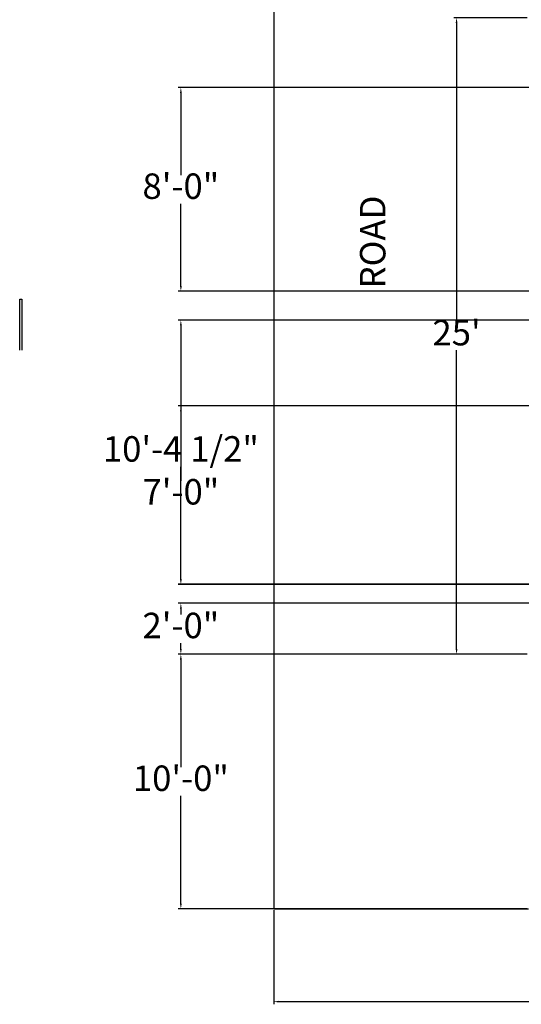
# Model space of a CAD drawing. Units: inches. Extents: x 5307 to 6359, y 4763 to 5474.
# Tile 1 of 5: x 5307 to 5543, y 4773 to 5237. Entities that reach past the tile are written whole.
import ezdxf

# ---------------------------------------------------------------- set-up
doc = ezdxf.new("R2010")
doc.units = ezdxf.units.IN
for name, color, linetype, lineweight in [('A-ANNO-DIMS', 2, 'Continuous', 18), ('A-ANNO-TEXT', 7, 'Continuous', 18), ('A-DOOR', 4, 'Continuous', 25), ('ROAD', 240, 'Continuous', 25)]:
    doc.layers.add(name, color=color, linetype=linetype, lineweight=lineweight)
doc.styles.get("Standard").update_dxf_attribs({"font": 'arial.ttf'})
doc.dimstyles.new('ISO-25', dxfattribs={"dimtxt": 12, "dimasz": 2.5, "dimexe": 1.25, "dimexo": 0.625, "dimtad": 1, "dimtih": 1, "dimtoh": 1, "dimlunit": 4, "dimtxsty": 'Standard', "dimcen": 2.5, "dimadec": 0, "dimazin": 0, "dimtfac": 1, "dimtmove": 0, "dimatfit": 3, "dimfxl": 1, "dimarcsym": 0})

# ---------------------------------------------------------------- blocks, each defined once
blk = doc.blocks.new('*D3')
at = {"layer": 'A-ANNO-DIMS', "color": 0, "lineweight": -2, "transparency": 16777216}
for p, q in [((5545.97, 5237.78), (5511.45, 5237.78)), ((5512.7, 5235.28), (5512.7, 5094.54)), ((5512.7, 4940.28), (5512.7, 5081.03)), ((5545.97, 4937.78), (5511.45, 4937.78))]:
    blk.add_line(p, q, dxfattribs=at)
at = {"layer": 'A-ANNO-DIMS', "color": 0, "transparency": 16777216}
for points in [[(5512.28, 5235.28), (5513.12, 5235.28), (5512.7, 5237.78)], [(5512.28, 4940.28), (5513.12, 4940.28), (5512.7, 4937.78)]]:
    blk.add_solid(points, dxfattribs=at)
at = {"layer": 'Defpoints', "color": 0, "transparency": 16777216}
for p in [(5546.59, 5237.78), (5512.7, 4937.78), (5546.59, 4937.78)]:
    blk.add_point(p, dxfattribs=at)
at = {"layer": 'A-ANNO-DIMS', "color": 0, "transparency": 16777216, "insert": (5512.7, 5087.78), "char_height": 12, "attachment_point": 5}
blk.add_mtext("25'", dxfattribs=at)
blk = doc.blocks.new('DOOR-LEAF-24IN')
for p, q in [((0, 0), (0, 24)), ((0, 24), (1, 24)), ((1, 24), (1, 0))]:
    blk.add_line(p, q)
blk = doc.blocks.new('*D12')
at = {"layer": 'A-ANNO-DIMS', "color": 0, "lineweight": -2, "transparency": 16777216}
for p, q in [((6038.59, 4937.16), (6038.59, 4772.78)), ((5426.59, 4817.16), (5426.59, 4772.78)), ((5429.09, 4774.03), (6036.09, 4774.03))]:
    blk.add_line(p, q, dxfattribs=at)
at = {"layer": 'A-ANNO-DIMS', "color": 0, "transparency": 16777216}
for points in [[(5429.09, 4774.45), (5429.09, 4773.62), (5426.59, 4774.03)], [(6036.09, 4774.45), (6036.09, 4773.62), (6038.59, 4774.03)]]:
    blk.add_solid(points, dxfattribs=at)
at = {"layer": 'Defpoints', "color": 0, "transparency": 16777216}
for p in [(6038.59, 4937.78), (5426.59, 4817.78), (6038.59, 4774.03)]:
    blk.add_point(p, dxfattribs=at)
at = {"layer": 'A-ANNO-DIMS', "color": 0, "transparency": 16777216, "insert": (5732.59, 4780.79), "char_height": 12, "attachment_point": 5}
blk.add_mtext('51\'-0"', dxfattribs=at)
blk = doc.blocks.new('*D15')
at = {"layer": 'A-ANNO-DIMS', "color": 0, "lineweight": -2, "transparency": 16777216}
for p, q in [((5569.97, 4961.78), (5381.59, 4961.78)), ((5382.84, 4959.28), (5382.84, 4956.54)), ((5382.84, 4940.28), (5382.84, 4943.03)), ((5545.97, 4937.78), (5381.59, 4937.78))]:
    blk.add_line(p, q, dxfattribs=at)
at = {"layer": 'A-ANNO-DIMS', "color": 0, "transparency": 16777216}
for points in [[(5382.43, 4959.28), (5383.26, 4959.28), (5382.84, 4961.78)], [(5382.43, 4940.28), (5383.26, 4940.28), (5382.84, 4937.78)]]:
    blk.add_solid(points, dxfattribs=at)
at = {"layer": 'Defpoints', "color": 0, "transparency": 16777216}
for p in [(5382.84, 4961.78), (5570.59, 4961.78), (5546.59, 4937.78)]:
    blk.add_point(p, dxfattribs=at)
at = {"layer": 'A-ANNO-DIMS', "color": 0, "transparency": 16777216, "insert": (5382.84, 4949.78), "char_height": 12, "attachment_point": 5}
blk.add_mtext('2\'-0"', dxfattribs=at)
blk = doc.blocks.new('*D18')
at = {"layer": 'A-ANNO-DIMS', "color": 0, "lineweight": -2, "transparency": 16777216}
for p, q in [((5545.97, 4937.78), (5381.59, 4937.78)), ((5382.84, 4935.28), (5382.84, 4884.54)), ((5382.84, 4820.28), (5382.84, 4871.03)), ((5545.97, 4817.78), (5381.59, 4817.78))]:
    blk.add_line(p, q, dxfattribs=at)
at = {"layer": 'A-ANNO-DIMS', "color": 0, "transparency": 16777216}
for points in [[(5382.43, 4935.28), (5383.26, 4935.28), (5382.84, 4937.78)], [(5382.43, 4820.28), (5383.26, 4820.28), (5382.84, 4817.78)]]:
    blk.add_solid(points, dxfattribs=at)
at = {"layer": 'Defpoints', "color": 0, "transparency": 16777216}
for p in [(5382.84, 4937.78), (5546.59, 4937.78), (5546.59, 4817.78)]:
    blk.add_point(p, dxfattribs=at)
at = {"layer": 'A-ANNO-DIMS', "color": 0, "transparency": 16777216, "insert": (5382.84, 4877.78), "char_height": 12, "attachment_point": 5}
blk.add_mtext('10\'-0"', dxfattribs=at)
blk = doc.blocks.new('*D27')
at = {"layer": 'A-ANNO-DIMS', "color": 0, "lineweight": -2, "transparency": 16777216}
for p, q in [((5578.97, 5054.78), (5381.59, 5054.78)), ((5382.84, 5052.28), (5382.84, 5019.54)), ((5382.84, 4973.28), (5382.84, 5006.03)), ((5578.97, 4970.78), (5381.59, 4970.78))]:
    blk.add_line(p, q, dxfattribs=at)
at = {"layer": 'A-ANNO-DIMS', "color": 0, "transparency": 16777216}
for points in [[(5382.43, 5052.28), (5383.26, 5052.28), (5382.84, 5054.78)], [(5382.43, 4973.28), (5383.26, 4973.28), (5382.84, 4970.78)]]:
    blk.add_solid(points, dxfattribs=at)
at = {"layer": 'Defpoints', "color": 0, "transparency": 16777216}
for p in [(5382.84, 5054.78), (5579.59, 5054.78), (5579.59, 4970.78)]:
    blk.add_point(p, dxfattribs=at)
at = {"layer": 'A-ANNO-DIMS', "color": 0, "transparency": 16777216, "insert": (5382.84, 5012.78), "char_height": 12, "attachment_point": 5}
blk.add_mtext('7\'-0"', dxfattribs=at)
blk = doc.blocks.new('*D28')
at = {"layer": 'A-ANNO-DIMS', "color": 0, "lineweight": -2, "transparency": 16777216}
for p, q in [((5578.97, 5204.82), (5381.59, 5204.82)), ((5382.84, 5202.32), (5382.84, 5163.57)), ((5382.84, 5111.32), (5382.84, 5150.06)), ((5578.97, 5108.82), (5381.59, 5108.82))]:
    blk.add_line(p, q, dxfattribs=at)
at = {"layer": 'A-ANNO-DIMS', "color": 0, "transparency": 16777216}
for points in [[(5382.43, 5202.32), (5383.26, 5202.32), (5382.84, 5204.82)], [(5382.43, 5111.32), (5383.26, 5111.32), (5382.84, 5108.82)]]:
    blk.add_solid(points, dxfattribs=at)
at = {"layer": 'Defpoints', "color": 0, "transparency": 16777216}
for p in [(5382.84, 5204.82), (5579.59, 5204.82), (5579.59, 5108.82)]:
    blk.add_point(p, dxfattribs=at)
at = {"layer": 'A-ANNO-DIMS', "color": 0, "transparency": 16777216, "insert": (5382.84, 5156.82), "char_height": 12, "attachment_point": 5}
blk.add_mtext('8\'-0"', dxfattribs=at)
blk = doc.blocks.new('*D29')
at = {"layer": 'A-ANNO-DIMS', "color": 0, "lineweight": -2, "transparency": 16777216}
for p, q in [((5904.31, 5095.28), (5381.59, 5095.28)), ((5382.84, 5092.78), (5382.84, 5039.81)), ((5382.84, 4973.19), (5382.84, 5026.16)), ((5904.44, 4970.69), (5381.59, 4970.69))]:
    blk.add_line(p, q, dxfattribs=at)
at = {"layer": 'A-ANNO-DIMS', "color": 0, "transparency": 16777216}
for points in [[(5382.43, 5092.78), (5383.26, 5092.78), (5382.84, 5095.28)], [(5382.43, 4973.19), (5383.26, 4973.19), (5382.84, 4970.69)]]:
    blk.add_solid(points, dxfattribs=at)
at = {"layer": 'Defpoints', "color": 0, "transparency": 16777216}
for p in [(5382.84, 5095.28), (5904.94, 5095.28), (5905.06, 4970.69)]:
    blk.add_point(p, dxfattribs=at)
at = {"layer": 'A-ANNO-DIMS', "color": 0, "transparency": 16777216, "insert": (5382.84, 5032.99), "char_height": 12, "attachment_point": 5}
blk.add_mtext('10\'-4 1/2"', dxfattribs=at)

msp = doc.modelspace()

# ---------------------------------------------------------------- linework, layer by layer
at = {"layer": 'ROAD'}
for p, q in [((5426.592, 5357.784), (5426.592, 4817.784)), ((5426.592, 4817.784), (5546.592, 4817.784))]:
    msp.add_line(p, q, dxfattribs=at)

# ---------------------------------------------------------------- block references
at = {"layer": 'A-DOOR'}
msp.add_blockref('DOOR-LEAF-24IN', (5306.929, 5081.064), dxfattribs=at)

# ---------------------------------------------------------------- texts
at = {"layer": 'A-ANNO-TEXT', "insert": (5467.207, 5110.187), "char_height": 12, "attachment_point": 1, "rotation": 90}
msp.add_mtext_dynamic_manual_height_columns('ROAD', width=33.49855, gutter_width=12.5, heights=[0], dxfattribs=at)

# ---------------------------------------------------------------- dimensions: what is measured, and where the dimension line sits
at = {"layer": 'A-ANNO-DIMS'}
for base, p1, p2, override, picture, middle in [((5512.7, 4937.784), (5546.592, 5237.784), (5546.592, 4937.784), {"dimclrd": 0, "dimclre": 0, "dimclrt": 0}, '*D3', (5512.7, 5087.784)), ((5382.842, 5204.816), (5579.592, 5108.816), (5579.592, 5204.816), {"dimdec": 1, "dimlfac": 1, "dimrnd": 0, "dimzin": 1, "dimdsep": 46, "dimlunit": 4, "dimfrac": 2}, '*D28', (5382.842, 5156.816)), ((5382.842, 5095.284), (5905.06, 4970.686), (5904.94, 5095.284), {"dimdec": 1, "dimlfac": 1, "dimrnd": 0, "dimzin": 1, "dimdsep": 46, "dimlunit": 4, "dimfrac": 2}, '*D29', (5382.842, 5032.985)), ((5382.842, 5054.784), (5579.592, 4970.784), (5579.592, 5054.784), {"dimdec": 1, "dimlfac": 1, "dimrnd": 0, "dimzin": 1, "dimdsep": 46, "dimlunit": 4, "dimfrac": 2}, '*D27', (5382.842, 5012.784)), ((5382.842, 4961.784), (5546.592, 4937.784), (5570.592, 4961.784), {"dimdec": 1, "dimlfac": 1, "dimrnd": 0, "dimzin": 1, "dimdsep": 46, "dimlunit": 4, "dimfrac": 2}, '*D15', (5382.842, 4949.784)), ((5382.842, 4937.784), (5546.592, 4817.784), (5546.592, 4937.784), {"dimdec": 1, "dimlfac": 1, "dimrnd": 0, "dimzin": 1, "dimdsep": 46, "dimlunit": 4, "dimfrac": 2}, '*D18', (5382.842, 4877.784))]:
    dim = msp.add_linear_dim(base=base, p1=p1, p2=p2, angle=90, dimstyle='ISO-25', override=override, dxfattribs=at)
    dim.commit()
    dim.dimension.update_dxf_attribs({"geometry": picture, "text_midpoint": middle})
dim = msp.add_linear_dim(base=(6038.592, 4774.034), p1=(5426.592, 4817.784), p2=(6038.592, 4937.784), dimstyle='ISO-25', override={"dimdec": 1, "dimlfac": 1, "dimrnd": 0, "dimzin": 1, "dimdsep": 46, "dimlunit": 4, "dimfrac": 2}, dxfattribs=at)
dim.commit()
dim.dimension.update_dxf_attribs({"geometry": '*D12', "text_midpoint": (5732.592, 4780.786)})

doc.saveas('drawing.dxf')
